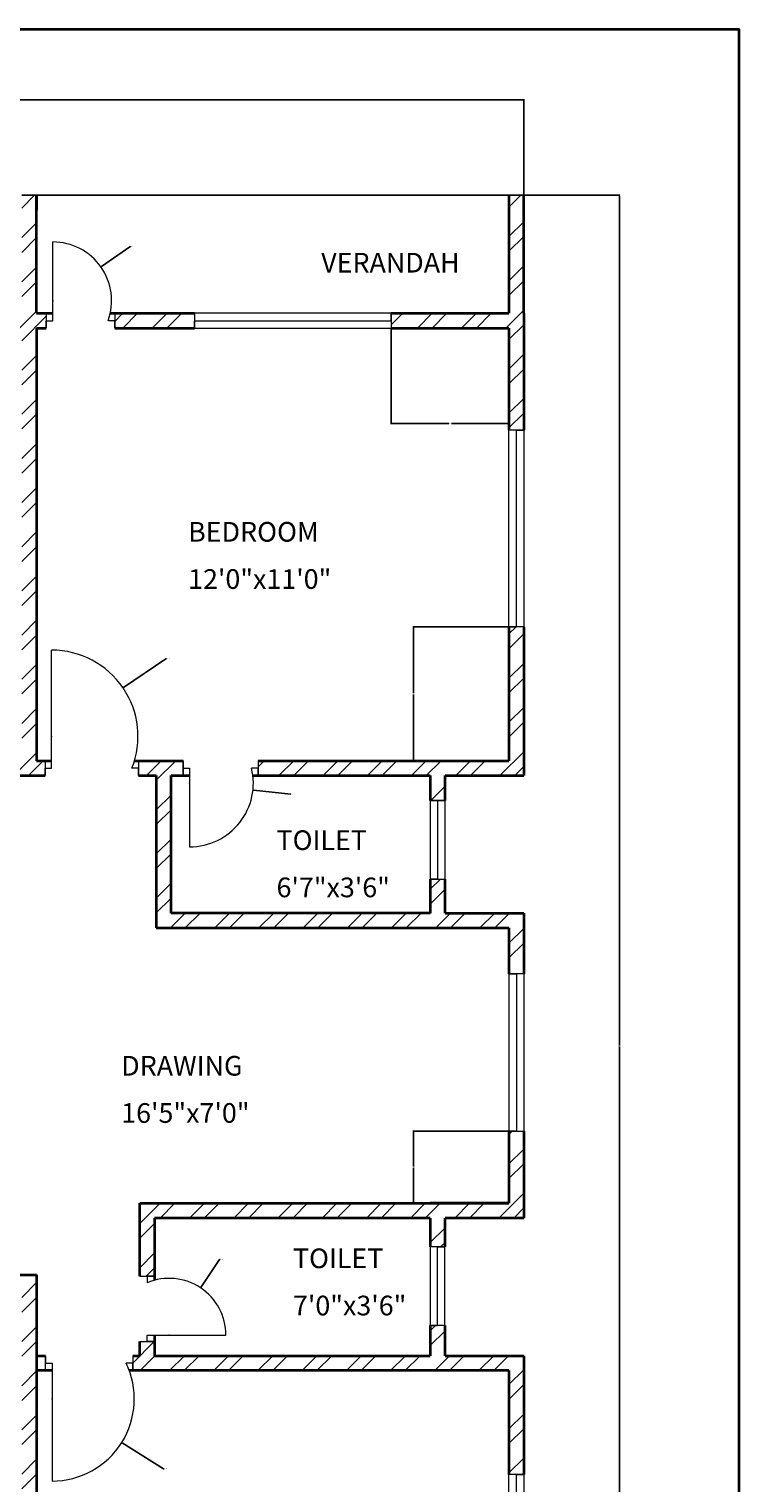
# Model space of a CAD drawing. Units: inches. Extents: x 2271 to 2815, y 1169 to 1838.
# Tile 4 of 4: x 2599 to 2815, y 1395 to 1838. Entities that reach past the tile are written whole.
import ezdxf

# ---------------------------------------------------------------- set-up
doc = ezdxf.new("R2010")
doc.units = ezdxf.units.IN
for name, color, linetype, lineweight in [('A-ANNO-DIMS', 2, 'Continuous', 18), ('A-ANNO-TTLB', 7, 'Continuous', 35), ('A-AREA-IDEN', 7, 'Continuous', 18), ('A-DOOR', 11, 'Continuous', 18), ('A-FLOR-EDGE', 7, 'Continuous', 25), ('A-GLAZ', 181, 'Continuous', 18), ('A-WALL', 7, 'Continuous', 35)]:
    doc.layers.add(name, color=color, linetype=linetype, lineweight=lineweight)
doc.layers.add('A-WALL-PATT', color=9, linetype='Continuous', lineweight=13, true_color=0xafd9aa)
doc.styles.get("Standard").update_dxf_attribs({"font": 'arial.ttf'})
doc.dimstyles.get("Standard").update_dxf_attribs({"dimtxt": 0.18, "dimasz": 0.18, "dimexe": 0.18, "dimexo": 0.0625, "dimgap": 0.09, "dimtad": 0, "dimtih": 1, "dimtoh": 1, "dimdec": 4, "dimzin": 0, "dimdsep": 46, "dimtxsty": 'Standard', "dimcen": 0.09, "dimadec": 0, "dimazin": 0, "dimtfac": 1, "dimtdec": 4, "dimtofl": 0, "dimtmove": 0, "dimatfit": 3, "dimfxl": 1, "dimtolj": 1, "dimtzin": 0, "dimarcsym": 0})

# ---------------------------------------------------------------- blocks, each defined once
blk = doc.blocks.new('WIN-60IN')
for p, q in [((0, 4.5), (0, 0)), ((60, 4.5), (0, 4.5)), ((60, 2.25), (60, 4.5)), ((60, 4.5), (60, 0)), ((0, 0), (0, 2.25)), ((0, 2.25), (60, 2.25)), ((0, 0), (60, 0))]:
    blk.add_line(p, q)
blk = doc.blocks.new('WIN-24IN')
for p, q in [((0, 4.5), (0, 0)), ((0, 4.5), (24, 4.5)), ((24, 2.25), (24, 4.5)), ((24, 4.5), (24, 0)), ((0, 0), (0, 2.25)), ((0, 2.25), (24, 2.25)), ((24, 0), (0, 0))]:
    blk.add_line(p, q)
blk = doc.blocks.new('*D7')
at = {"layer": 'A-ANNO-DIMS', "color": 0, "lineweight": -2, "transparency": 16777216}
for p, q in [((2318.8, 1787.59), (2318.8, 1816.86)), ((2318.98, 1816.68), (2533.65, 1816.68)), ((2749.12, 1816.68), (2534.45, 1816.68)), ((2749.3, 1787.59), (2749.3, 1816.86))]:
    blk.add_line(p, q, dxfattribs=at)
at = {"layer": 'A-ANNO-DIMS', "color": 0, "transparency": 16777216}
for points in [[(2318.98, 1816.71), (2318.98, 1816.65), (2318.8, 1816.68)], [(2749.12, 1816.71), (2749.12, 1816.65), (2749.3, 1816.68)]]:
    blk.add_solid(points, dxfattribs=at)
at = {"layer": 'Defpoints', "color": 0, "transparency": 16777216}
for p in [(2749.3, 1816.68), (2318.8, 1787.53), (2749.3, 1787.53)]:
    blk.add_point(p, dxfattribs=at)
at = {"layer": 'A-ANNO-DIMS', "color": 0, "transparency": 16777216, "insert": (2534.05, 1816.68), "char_height": 0.18, "attachment_point": 5}
blk.add_mtext('\\A1;430.5', dxfattribs=at)
blk = doc.blocks.new('*D8')
at = {"layer": 'A-ANNO-DIMS', "color": 0, "lineweight": -2, "transparency": 16777216}
for p, q in [((2749.36, 1787.53), (2778.63, 1787.53)), ((2778.45, 1787.35), (2778.45, 1528.21)), ((2778.45, 1268.71), (2778.45, 1527.85)), ((2749.36, 1268.53), (2778.63, 1268.53))]:
    blk.add_line(p, q, dxfattribs=at)
at = {"layer": 'A-ANNO-DIMS', "color": 0, "transparency": 16777216}
for points in [[(2778.42, 1787.35), (2778.48, 1787.35), (2778.45, 1787.53)], [(2778.42, 1268.71), (2778.48, 1268.71), (2778.45, 1268.53)]]:
    blk.add_solid(points, dxfattribs=at)
at = {"layer": 'Defpoints', "color": 0, "transparency": 16777216}
for p in [(2749.3, 1787.53), (2778.45, 1787.53), (2749.3, 1268.53)]:
    blk.add_point(p, dxfattribs=at)
at = {"layer": 'A-ANNO-DIMS', "color": 0, "transparency": 16777216, "insert": (2778.45, 1528.03), "char_height": 0.18, "attachment_point": 5}
blk.add_mtext('\\A1;519', dxfattribs=at)
blk = doc.blocks.new('*D29')
at = {"layer": 'A-ANNO-DIMS', "color": 0, "lineweight": -2, "transparency": 16777216}
for p, q in [((2708.93, 1746.97), (2708.93, 1717.7)), ((2744.8, 1746.97), (2744.8, 1717.7)), ((2709.11, 1717.88), (2726.47, 1717.88)), ((2744.62, 1717.88), (2727.26, 1717.88))]:
    blk.add_line(p, q, dxfattribs=at)
at = {"layer": 'A-ANNO-DIMS', "color": 0, "transparency": 16777216}
for points in [[(2709.11, 1717.91), (2709.11, 1717.85), (2708.93, 1717.88)], [(2744.62, 1717.91), (2744.62, 1717.85), (2744.8, 1717.88)]]:
    blk.add_solid(points, dxfattribs=at)
at = {"layer": 'Defpoints', "color": 0, "transparency": 16777216}
for p in [(2708.93, 1747.03), (2744.8, 1747.03), (2708.93, 1717.88)]:
    blk.add_point(p, dxfattribs=at)
at = {"layer": 'A-ANNO-DIMS', "color": 0, "transparency": 16777216, "insert": (2726.87, 1717.88), "char_height": 0.18, "attachment_point": 5}
blk.add_mtext('\\A1;35.87', dxfattribs=at)
blk = doc.blocks.new('*D34')
at = {"layer": 'A-ANNO-DIMS', "color": 0, "lineweight": -2, "transparency": 16777216}
for p, q in [((2744.74, 1655.86), (2715.47, 1655.86)), ((2715.65, 1655.68), (2715.65, 1635.63)), ((2715.65, 1615.21), (2715.65, 1635.26)), ((2744.74, 1615.03), (2715.47, 1615.03))]:
    blk.add_line(p, q, dxfattribs=at)
at = {"layer": 'A-ANNO-DIMS', "color": 0, "transparency": 16777216}
for points in [[(2715.62, 1655.68), (2715.68, 1655.68), (2715.65, 1655.86)], [(2715.62, 1615.21), (2715.68, 1615.21), (2715.65, 1615.03)]]:
    blk.add_solid(points, dxfattribs=at)
at = {"layer": 'Defpoints', "color": 0, "transparency": 16777216}
for p in [(2715.65, 1655.86), (2744.8, 1655.86), (2744.8, 1615.03)]:
    blk.add_point(p, dxfattribs=at)
at = {"layer": 'A-ANNO-DIMS', "color": 0, "transparency": 16777216, "insert": (2715.65, 1635.44), "char_height": 0.18, "attachment_point": 5}
blk.add_mtext('\\A1;40.826', dxfattribs=at)
blk = doc.blocks.new('*D35')
at = {"layer": 'A-ANNO-DIMS', "color": 0, "lineweight": -2, "transparency": 16777216}
for p, q in [((2744.74, 1502.04), (2715.47, 1502.04)), ((2715.65, 1501.86), (2715.65, 1491.22)), ((2715.65, 1480.21), (2715.65, 1490.85)), ((2744.74, 1480.03), (2715.47, 1480.03))]:
    blk.add_line(p, q, dxfattribs=at)
at = {"layer": 'A-ANNO-DIMS', "color": 0, "transparency": 16777216}
for points in [[(2715.62, 1501.86), (2715.68, 1501.86), (2715.65, 1502.04)], [(2715.62, 1480.21), (2715.68, 1480.21), (2715.65, 1480.03)]]:
    blk.add_solid(points, dxfattribs=at)
at = {"layer": 'Defpoints', "color": 0, "transparency": 16777216}
for p in [(2715.65, 1502.04), (2744.8, 1502.04), (2744.8, 1480.03)]:
    blk.add_point(p, dxfattribs=at)
at = {"layer": 'A-ANNO-DIMS', "color": 0, "transparency": 16777216, "insert": (2715.65, 1491.04), "char_height": 0.18, "attachment_point": 5}
blk.add_mtext('\\A1;22.01', dxfattribs=at)
blk = doc.blocks.new('*D40')
at = {"layer": 'A-ANNO-DIMS', "color": 0, "lineweight": -2, "transparency": 16777216}
for p, q in [((2640.24, 1646.14), (2627.33, 1637.36)), ((2640.42, 1646.14), (2640.24, 1646.14)), ((2605.33, 1622.46), (2605.51, 1622.46)), ((2605.42, 1622.37), (2605.42, 1622.55))]:
    blk.add_line(p, q, dxfattribs=at)
at = {"layer": 'A-ANNO-DIMS', "color": 0, "transparency": 16777216}
blk.add_solid([(2627.31, 1637.39), (2627.35, 1637.34), (2627.18, 1637.26)], dxfattribs=at)
at = {"layer": 'Defpoints', "color": 0, "transparency": 16777216}
for p in [(2627.18, 1637.26), (2605.42, 1622.46)]:
    blk.add_point(p, dxfattribs=at)
at = {"layer": 'A-ANNO-DIMS', "color": 0, "transparency": 16777216, "insert": (2640.9, 1646.14), "char_height": 0.18, "attachment_point": 5}
blk.add_mtext('\\A1;R26.32', dxfattribs=at)
blk = doc.blocks.new('*D42')
at = {"layer": 'A-ANNO-DIMS', "color": 0, "lineweight": -2, "transparency": 16777216}
for p, q in [((2605.45, 1420.36), (2605.63, 1420.36)), ((2605.54, 1420.27), (2605.54, 1420.45)), ((2639.53, 1399.04), (2626.94, 1406.94)), ((2639.71, 1399.04), (2639.53, 1399.04))]:
    blk.add_line(p, q, dxfattribs=at)
at = {"layer": 'A-ANNO-DIMS', "color": 0, "transparency": 16777216}
blk.add_solid([(2626.95, 1406.97), (2626.92, 1406.92), (2626.78, 1407.04)], dxfattribs=at)
at = {"layer": 'Defpoints', "color": 0, "transparency": 16777216}
for p in [(2605.54, 1420.36), (2626.78, 1407.04)]:
    blk.add_point(p, dxfattribs=at)
at = {"layer": 'A-ANNO-DIMS', "color": 0, "transparency": 16777216, "insert": (2640.19, 1399.04), "char_height": 0.18, "attachment_point": 5}
blk.add_mtext('\\A1;R25.08', dxfattribs=at)
blk = doc.blocks.new('*D44')
at = {"layer": 'A-ANNO-DIMS', "color": 0, "lineweight": -2, "transparency": 16777216}
for p, q in [((2647.39, 1608.19), (2647.57, 1608.19)), ((2647.48, 1608.1), (2647.48, 1608.28)), ((2678.36, 1604.85), (2666.96, 1606.08))]:
    blk.add_line(p, q, dxfattribs=at)
at = {"layer": 'A-ANNO-DIMS', "color": 0, "transparency": 16777216}
blk.add_solid([(2666.96, 1606.11), (2666.96, 1606.05), (2666.78, 1606.1)], dxfattribs=at)
at = {"layer": 'Defpoints', "color": 0, "transparency": 16777216}
for p in [(2647.48, 1608.19), (2666.78, 1606.1)]:
    blk.add_point(p, dxfattribs=at)
at = {"layer": 'A-ANNO-DIMS', "color": 0, "transparency": 16777216, "insert": (2678.91, 1604.85), "char_height": 0.18, "attachment_point": 5}
blk.add_mtext('\\A1;R19.413', dxfattribs=at)
blk = doc.blocks.new('*D48')
at = {"layer": 'A-ANNO-DIMS', "color": 0, "lineweight": -2, "transparency": 16777216}
for p, q in [((2629.25, 1771.84), (2620.6, 1765.76)), ((2629.43, 1771.84), (2629.25, 1771.84)), ((2605.7, 1755.37), (2605.88, 1755.37)), ((2605.79, 1755.28), (2605.79, 1755.46))]:
    blk.add_line(p, q, dxfattribs=at)
at = {"layer": 'A-ANNO-DIMS', "color": 0, "transparency": 16777216}
blk.add_solid([(2620.58, 1765.79), (2620.62, 1765.74), (2620.45, 1765.66)], dxfattribs=at)
at = {"layer": 'Defpoints', "color": 0, "transparency": 16777216}
for p in [(2620.45, 1765.66), (2605.79, 1755.37)]:
    blk.add_point(p, dxfattribs=at)
at = {"layer": 'A-ANNO-DIMS', "color": 0, "transparency": 16777216, "insert": (2629.98, 1771.84), "char_height": 0.18, "attachment_point": 5}
blk.add_mtext('\\A1;R17.915', dxfattribs=at)
blk = doc.blocks.new('*D50')
at = {"layer": 'A-ANNO-DIMS', "color": 0, "lineweight": -2, "transparency": 16777216}
for p, q in [((2656.58, 1462.88), (2650.93, 1454.39)), ((2656.76, 1462.88), (2656.58, 1462.88)), ((2641.16, 1439.83), (2641.34, 1439.83)), ((2641.25, 1439.74), (2641.25, 1439.92))]:
    blk.add_line(p, q, dxfattribs=at)
at = {"layer": 'A-ANNO-DIMS', "color": 0, "transparency": 16777216}
blk.add_solid([(2650.9, 1454.41), (2650.95, 1454.37), (2650.83, 1454.24)], dxfattribs=at)
at = {"layer": 'Defpoints', "color": 0, "transparency": 16777216}
for p in [(2650.83, 1454.24), (2641.25, 1439.83)]:
    blk.add_point(p, dxfattribs=at)
at = {"layer": 'A-ANNO-DIMS', "color": 0, "transparency": 16777216, "insert": (2657.3, 1462.88), "char_height": 0.18, "attachment_point": 5}
blk.add_mtext('\\A1;R17.304', dxfattribs=at)

msp = doc.modelspace()

# ---------------------------------------------------------------- hatches: boundary and pattern name
at = {"layer": 'A-WALL-PATT'}
h = msp.add_hatch(dxfattribs=at)
h.set_pattern_fill('ANSI32', color=256)
h.paths.add_polyline_path([(2441.4917, 1751.5314), (2397.0578, 1751.5314), (2397.0578, 1747.0314), (2441.4917, 1747.0314), (2441.4917, 1749.2814)])
h.paths.add_polyline_path([(2471.8006, 1787.5314), (2467.3006, 1787.5314), (2467.3006, 1783.0314), (2467.3006, 1751.5314), (2463.4131, 1751.5314), (2463.4131, 1747.0314), (2467.3006, 1747.0314), (2467.3006, 1615.0314), (2465.0606, 1615.0314), (2465.0606, 1610.5314), (2474.7192, 1610.5314), (2474.7192, 1612.7814), (2474.7192, 1615.0314), (2471.8006, 1615.0314), (2471.8006, 1747.0314), (2482.8275, 1747.0314), (2482.8275, 1749.2814), (2482.8275, 1751.5314), (2471.8006, 1751.5314)])
h.paths.add_polyline_path([(2549.5185, 1751.5314), (2506.8275, 1751.5314), (2506.8275, 1747.0314), (2531.8006, 1747.0314), (2531.8006, 1615.0314), (2496.0724, 1615.0314), (2496.0724, 1610.5314), (2531.8006, 1610.5314), (2531.8006, 1458.2548), (2528.7405, 1458.2548), (2528.7405, 1453.7548), (2539.7806, 1453.7548), (2539.7806, 1456.0048), (2539.7806, 1458.2548), (2536.3006, 1458.2548), (2536.3006, 1610.5314), (2573.267, 1610.5314), (2573.267, 1612.5736), (2573.267, 1612.7912), (2573.267, 1615.0314), (2536.3006, 1615.0314), (2536.3006, 1747.0314), (2549.5185, 1747.0314)])
h.paths.add_polyline_path([(2600.8006, 1787.5314), (2596.3006, 1787.5314), (2596.3006, 1747.0314), (2596.3006, 1615.0314), (2593.1473, 1615.0314), (2593.1473, 1610.5314), (2603.416, 1610.5314), (2603.416, 1612.7814), (2603.416, 1615.0314), (2600.8006, 1615.0314), (2600.8006, 1747.0314), (2603.7892, 1747.0314), (2603.7892, 1749.2814), (2603.7892, 1751.5314), (2600.8006, 1751.5314)])
h.paths.add_polyline_path([(2596.3006, 1751.5314), (2573.5185, 1751.5314), (2573.5185, 1747.0314), (2596.3006, 1747.0314)])
h.paths.add_polyline_path([(2648.9302, 1749.2814), (2648.9302, 1751.5314), (2624.6394, 1751.5314), (2624.6394, 1747.0314), (2648.9302, 1747.0314)])
h.paths.add_polyline_path([(2749.3006, 1751.5314), (2749.3006, 1787.5314), (2744.8006, 1787.5314), (2744.8006, 1751.5314), (2708.9302, 1751.5314), (2708.9302, 1747.0314), (2744.8006, 1747.0314), (2744.8006, 1715.8571), (2749.3006, 1715.8571)])
h.paths.add_polyline_path([(2337.0578, 1749.2814), (2337.0578, 1751.5314), (2323.3006, 1751.5314), (2323.3006, 1787.5314), (2318.8006, 1787.5314), (2318.8006, 1751.5314), (2318.8006, 1712.2179), (2323.3006, 1712.2179), (2323.3006, 1747.0314), (2337.0578, 1747.0314)])
h.paths.add_polyline_path([(2402.757, 1615.0314), (2323.3006, 1615.0314), (2323.3006, 1652.2179), (2318.8006, 1652.2179), (2318.8006, 1610.5314), (2323.3006, 1610.5314), (2342.8006, 1610.5314), (2342.8006, 1602.42), (2347.3006, 1602.42), (2347.3006, 1610.5314), (2402.757, 1610.5314)])
h.paths.add_polyline_path([(2430.8006, 1568.5314), (2430.8006, 1610.5314), (2434.8435, 1610.5314), (2434.8435, 1612.7814), (2434.8435, 1615.0314), (2422.3947, 1615.0314), (2422.3947, 1612.7814), (2422.3947, 1610.5314), (2426.3006, 1610.5314), (2426.3006, 1568.5314), (2347.3006, 1568.5314), (2347.3006, 1578.42), (2342.8006, 1578.42), (2342.8006, 1568.5314), (2318.8006, 1568.5314), (2318.8006, 1546.0693), (2322.7121, 1546.0693), (2323.3006, 1546.0693), (2323.3006, 1564.0314), (2342.8006, 1564.0314), (2347.3006, 1564.0314), (2430.8006, 1564.0314)])
h.paths.add_polyline_path([(2430.8006, 1480.0314), (2323.3006, 1480.0314), (2323.3006, 1498.0693), (2321.0506, 1498.0693), (2318.8006, 1498.0693), (2318.8006, 1475.5314), (2342.8006, 1475.5314), (2342.8006, 1466.8218), (2347.3006, 1466.8218), (2347.3006, 1475.5314), (2426.3006, 1475.5314), (2426.3006, 1458.0149), (2430.8006, 1458.0149), (2430.8006, 1475.5314)])
h.paths.add_polyline_path([(2435.9471, 1433.5314), (2430.8006, 1433.5314), (2430.8006, 1437.7896), (2426.3006, 1437.7896), (2426.3006, 1433.5314), (2347.3006, 1433.5314), (2347.3006, 1442.8218), (2342.8006, 1442.8218), (2342.8006, 1433.5314), (2318.8006, 1433.5314), (2318.8006, 1402.3145), (2323.3006, 1402.3145), (2323.3006, 1429.0314), (2342.8006, 1429.0314), (2347.3006, 1429.0314), (2435.9471, 1429.0314)])
h.paths.add_polyline_path([(2323.3006, 1342.3145), (2321.0506, 1342.3145), (2318.8006, 1342.3145), (2318.8006, 1304.5314), (2318.8006, 1268.5314), (2323.3006, 1268.5314), (2323.3006, 1304.5314), (2333.4662, 1304.5314), (2333.4662, 1306.7814), (2333.4662, 1309.0314), (2323.3006, 1309.0314)])
h.paths.add_polyline_path([(2437.8933, 1306.7814), (2437.8933, 1309.0314), (2393.4662, 1309.0314), (2393.4662, 1304.5314), (2437.8933, 1304.5314)])
h.paths.add_polyline_path([(2471.8006, 1453.7548), (2493.7895, 1453.7548), (2493.7895, 1456.0048), (2493.7895, 1458.2548), (2467.3006, 1458.2548), (2467.3006, 1433.5314), (2463.7134, 1433.5314), (2463.7134, 1431.2814), (2463.7134, 1429.0314), (2467.3006, 1429.0314), (2467.3006, 1309.0314), (2462.3197, 1309.0314), (2462.3197, 1304.5314), (2467.3006, 1304.5314), (2467.3006, 1268.5314), (2471.8006, 1268.5314), (2495.9201, 1268.5314), (2495.9201, 1270.7814), (2495.9201, 1273.0314), (2471.8006, 1273.0314), (2471.8006, 1309.0314)])
h.paths.add_polyline_path([(2600.8006, 1458.2548), (2570.4818, 1458.2548), (2570.4818, 1453.7548), (2596.3006, 1453.7548), (2596.3006, 1429.0314), (2596.3006, 1273.0314), (2555.9201, 1273.0314), (2555.9201, 1268.5314), (2596.3006, 1268.5314), (2600.8006, 1268.5314), (2600.8006, 1304.5314), (2604.5593, 1304.5314), (2604.5593, 1306.7814), (2604.5593, 1309.0314), (2600.8006, 1309.0314), (2600.8006, 1429.0314)])
h.paths.add_polyline_path([(2667.0861, 1309.0314), (2627.2, 1309.0314), (2627.2, 1304.5314), (2667.0861, 1304.5314)])
h.paths.add_polyline_path([(2749.3006, 1309.0314), (2749.3006, 1337.3095), (2744.8006, 1337.3095), (2744.8006, 1309.0314), (2727.0861, 1309.0314), (2727.0861, 1306.7814), (2727.0861, 1304.5314), (2744.8006, 1304.5314), (2744.8006, 1268.5314), (2749.3006, 1268.5314), (2749.3006, 1304.5314)])
h.paths.add_polyline_path([(2749.3006, 1433.5314), (2725.3006, 1433.5314), (2725.3006, 1442.7202), (2720.8006, 1442.7202), (2720.8006, 1433.5314), (2636.8006, 1433.5314), (2636.8006, 1437.8287), (2634.5506, 1437.8287), (2632.3006, 1437.8287), (2632.3006, 1433.5314), (2630.1129, 1433.5314), (2630.1129, 1429.0314), (2744.8006, 1429.0314), (2744.8006, 1397.3095), (2749.3006, 1397.3095)])
h.paths.add_polyline_path([(2749.3006, 1480.0314), (2749.3006, 1502.0415), (2744.8006, 1502.0415), (2744.8006, 1480.0314), (2720.8006, 1480.0314), (2632.3006, 1480.0314), (2632.3006, 1457.7851), (2636.8006, 1457.7851), (2636.8006, 1475.5314), (2720.8006, 1475.5314), (2720.8006, 1466.7202), (2725.3006, 1466.7202), (2725.3006, 1475.5314), (2749.3006, 1475.5314)])
h.paths.add_polyline_path([(2749.3006, 1568.5314), (2725.3006, 1568.5314), (2725.3006, 1578.9125), (2720.8006, 1578.9125), (2720.8006, 1568.5314), (2641.8006, 1568.5314), (2641.8006, 1610.5314), (2645.4823, 1610.5314), (2645.4823, 1612.7814), (2645.4823, 1615.0314), (2631.895, 1615.0314), (2631.895, 1610.5314), (2637.3006, 1610.5314), (2637.3006, 1568.5314), (2637.3006, 1564.0314), (2720.8006, 1564.0314), (2725.3006, 1564.0314), (2744.8006, 1564.0314), (2744.8006, 1550.0415), (2747.0506, 1550.0415), (2749.3006, 1550.0415)])
h.paths.add_polyline_path([(2749.3006, 1655.8571), (2744.8006, 1655.8571), (2744.8006, 1615.0314), (2668.3453, 1615.0314), (2668.3453, 1610.5314), (2720.8006, 1610.5314), (2720.8006, 1602.9125), (2725.3006, 1602.9125), (2725.3006, 1610.5314), (2749.3006, 1610.5314)])
h.paths.add_polyline_path([(2512.9815, 1676.2212), (2512.9815, 1716.3099), (2486.1477, 1716.3099), (2486.1477, 1676.2212)], flags=9)

# ---------------------------------------------------------------- linework, layer by layer
at = {"layer": 'A-ANNO-TTLB'}
msp.add_lwpolyline([(2270.5512, 1838.2339), (2814.8691, 1838.2339), (2814.8691, 1168.8883), (2270.5512, 1168.8883)], close=True, dxfattribs=at)
at = {"layer": 'A-DOOR'}
for p, q in [((2605.7892, 1749.2814), (2605.7892, 1773.2814)), ((2603.7892, 1751.5314), (2603.7892, 1747.0314)), ((2603.7892, 1747.0314), (2603.7892, 1749.2814)), ((2603.7892, 1749.2814), (2605.7892, 1749.2814)), ((2624.6394, 1749.2814), (2622.6394, 1749.2814)), ((2624.6394, 1751.5314), (2624.6394, 1747.0314)), ((2624.6394, 1747.0314), (2624.6394, 1749.2814)), ((2605.416, 1612.7814), (2605.416, 1648.7814)), ((2603.416, 1615.0314), (2603.416, 1610.5314)), ((2631.895, 1615.0314), (2631.895, 1610.5314)), ((2645.4823, 1610.5314), (2645.4823, 1615.0314)), ((2645.4823, 1615.0314), (2645.4823, 1610.5314)), ((2668.3453, 1615.0314), (2668.3453, 1610.5314)), ((2603.416, 1610.5314), (2603.416, 1612.7814)), ((2603.416, 1612.7814), (2605.416, 1612.7814)), ((2631.895, 1612.7814), (2629.895, 1612.7814)), ((2631.895, 1610.5314), (2631.895, 1612.7814)), ((2645.4823, 1610.5314), (2645.4823, 1612.7814)), ((2645.4823, 1612.7814), (2647.4823, 1612.7814)), ((2647.4823, 1612.7814), (2647.4823, 1588.7814)), ((2668.3453, 1612.7814), (2666.3453, 1612.7814)), ((2668.3453, 1610.5314), (2668.3453, 1612.7814)), ((2632.3006, 1457.7851), (2636.8006, 1457.7851)), ((2636.8006, 1457.7851), (2634.5506, 1457.7851)), ((2634.5506, 1457.7851), (2634.5506, 1455.7851)), ((2632.3006, 1437.8287), (2636.8006, 1437.8287)), ((2634.5506, 1437.8287), (2634.5506, 1439.8287)), ((2634.5506, 1439.8287), (2658.5506, 1439.8287)), ((2636.8006, 1437.8287), (2634.5506, 1437.8287)), ((2603.5387, 1429.0314), (2603.5387, 1433.5314)), ((2603.5387, 1433.5314), (2603.5387, 1431.2814)), ((2630.1129, 1433.5314), (2630.1129, 1429.0314)), ((2603.5387, 1431.2814), (2605.5387, 1431.2814)), ((2605.5387, 1431.2814), (2605.5387, 1395.2814)), ((2630.1129, 1431.2814), (2628.1129, 1431.2814)), ((2630.1129, 1429.0314), (2630.1129, 1431.2814))]:
    msp.add_line(p, q, dxfattribs=at)
for centre, radius, start, end in [((2605.7892, 1755.3662), 17.9152, 340.144636, 90), ((2605.416, 1622.4589), 26.3225, 338.429293, 90), ((2647.4823, 1608.1941), 19.4127, 270, 13.668434), ((2641.2463, 1439.8287), 17.3043, 0, 112.764112), ((2605.5387, 1420.3591), 25.0777, 270, 25.819443)]:
    msp.add_arc(centre, radius, start, end, dxfattribs=at)
at = {"layer": 'A-FLOR-EDGE'}
msp.add_line((2749.3006, 1787.5314), (2596.3006, 1787.5314), dxfattribs=at)
at = {"layer": 'A-GLAZ'}
for p, q in [((2725.3006, 1602.9125), (2720.8006, 1602.9125)), ((2720.8006, 1602.9125), (2725.3006, 1602.9125)), ((2720.8006, 1602.9125), (2720.8006, 1578.9125)), ((2725.3006, 1602.9125), (2723.0506, 1602.9125)), ((2723.0506, 1602.9125), (2723.0506, 1578.9125)), ((2725.3006, 1578.9125), (2725.3006, 1602.9125)), ((2723.0506, 1578.9125), (2720.8006, 1578.9125)), ((2720.8006, 1578.9125), (2725.3006, 1578.9125)), ((2749.3006, 1550.0415), (2744.8006, 1550.0415)), ((2744.8006, 1550.0415), (2747.0506, 1550.0415)), ((2744.8006, 1550.0415), (2744.8006, 1502.0415)), ((2747.0506, 1550.0415), (2747.0506, 1502.0415)), ((2749.3006, 1550.0415), (2749.3006, 1502.0415)), ((2747.0506, 1502.0415), (2744.8006, 1502.0415)), ((2744.8006, 1502.0415), (2749.3006, 1502.0415))]:
    msp.add_line(p, q, dxfattribs=at)
at = {"layer": 'A-WALL'}
for p, q in [((2600.8006, 1751.5314), (2600.8006, 1787.5314)), ((2600.8006, 1787.5314), (2600.8006, 1783.0314)), ((2744.8006, 1787.5314), (2744.8006, 1751.5314)), ((2749.3006, 1751.5314), (2749.3006, 1787.5314)), ((2600.8006, 1751.5314), (2605.7892, 1751.5314)), ((2623.2892, 1751.5314), (2648.9302, 1751.5314)), ((2708.9302, 1751.5314), (2744.8006, 1751.5314)), ((2749.3006, 1751.5314), (2749.3006, 1715.8571)), ((2600.8006, 1747.0314), (2600.8006, 1615.0314)), ((2600.8006, 1747.0314), (2603.7892, 1747.0314)), ((2624.6394, 1747.0314), (2648.9302, 1747.0314)), ((2708.9302, 1747.0314), (2744.8006, 1747.0314)), ((2744.8006, 1747.0314), (2744.8006, 1715.8571)), ((2744.8006, 1655.8571), (2744.8006, 1615.0314)), ((2749.3006, 1655.8571), (2749.3006, 1610.5314)), ((2600.8006, 1615.0314), (2605.416, 1615.0314)), ((2630.6689, 1615.0314), (2645.4823, 1615.0314)), ((2668.3453, 1615.0314), (2744.8006, 1615.0314)), ((2593.1473, 1610.5314), (2603.416, 1610.5314)), ((2631.895, 1610.5314), (2637.3006, 1610.5314)), ((2637.3006, 1610.5314), (2637.3006, 1568.5314)), ((2641.8006, 1568.5314), (2641.8006, 1610.5314)), ((2641.8006, 1610.5314), (2647.4823, 1610.5314)), ((2666.7538, 1610.5314), (2720.8006, 1610.5314)), ((2720.8006, 1610.5314), (2720.8006, 1602.9125)), ((2720.8006, 1610.5314), (2720.8006, 1602.9125)), ((2725.3006, 1610.5314), (2749.3006, 1610.5314)), ((2725.3006, 1602.9125), (2725.3006, 1610.5314)), ((2720.8006, 1578.9125), (2720.8006, 1568.5314)), ((2720.8006, 1578.9125), (2720.8006, 1568.5314)), ((2725.3006, 1568.5314), (2725.3006, 1578.9125)), ((2637.3006, 1568.5314), (2637.3006, 1564.0314)), ((2720.8006, 1568.5314), (2641.8006, 1568.5314)), ((2725.3006, 1568.5314), (2749.3006, 1568.5314)), ((2749.3006, 1568.5314), (2749.3006, 1550.0415)), ((2637.3006, 1564.0314), (2720.8006, 1564.0314)), ((2720.8006, 1564.0314), (2720.8006, 1564.0314)), ((2720.8006, 1564.0314), (2725.3006, 1564.0314)), ((2725.3006, 1564.0314), (2744.8006, 1564.0314)), ((2744.8006, 1564.0314), (2744.8006, 1550.0415)), ((2744.8006, 1502.0415), (2744.8006, 1480.0314)), ((2749.3006, 1502.0415), (2749.3006, 1475.5314)), ((2632.3006, 1480.0314), (2744.8006, 1480.0314)), ((2632.3006, 1457.7851), (2632.3006, 1480.0314)), ((2744.8006, 1480.0314), (2720.8006, 1480.0314)), ((2749.3006, 1480.0314), (2749.3006, 1475.5314)), ((2720.8006, 1475.5314), (2636.8006, 1475.5314)), ((2636.8006, 1475.5314), (2636.8006, 1456.5521)), ((2720.8006, 1475.5314), (2720.8006, 1466.7202)), ((2749.3006, 1475.5314), (2725.3006, 1475.5314)), ((2725.3006, 1466.7202), (2725.3006, 1475.5314)), ((2569.063, 1458.2548), (2600.8006, 1458.2548)), ((2600.8006, 1458.2548), (2600.8006, 1429.0314)), ((2720.8006, 1442.7202), (2720.8006, 1433.5314)), ((2725.3006, 1433.5314), (2725.3006, 1442.7202)), ((2632.3006, 1433.5314), (2632.3006, 1437.8287)), ((2636.8006, 1439.8287), (2636.8006, 1433.5314)), ((2600.8006, 1433.5314), (2603.5387, 1433.5314)), ((2630.1129, 1433.5314), (2632.3006, 1433.5314)), ((2636.8006, 1433.5314), (2720.8006, 1433.5314)), ((2725.3006, 1433.5314), (2749.3006, 1433.5314)), ((2749.3006, 1433.5314), (2749.3006, 1397.3095)), ((2600.8006, 1429.0314), (2600.8006, 1309.0314)), ((2605.5387, 1429.0314), (2600.8006, 1429.0314)), ((2744.8006, 1429.0314), (2629.0692, 1429.0314)), ((2744.8006, 1429.0314), (2744.8006, 1397.3095))]:
    msp.add_line(p, q, dxfattribs=at)

# ---------------------------------------------------------------- block references
at = {"layer": 'A-GLAZ'}
msp.add_blockref('WIN-60IN', (2648.9304, 1747.031), dxfattribs=at)
at = {"layer": 'A-GLAZ', "extrusion": (0, 0, -1), "zscale": -1, "rotation": 90}
for name, p in [('WIN-60IN', (-2744.8001, 1655.8574)), ('WIN-24IN', (-2720.8001, 1442.7197)), ('WIN-60IN', (-2744.8001, 1337.3097))]:
    msp.add_blockref(name, p, dxfattribs=at)

# ---------------------------------------------------------------- texts
at = {"layer": 'A-AREA-IDEN', "char_height": 6, "attachment_point": 1, "line_spacing_factor": 1.44}
for s, width, insert in [('VERANDAH', 202.405664, (2687.575, 1769.9702)), ('BEDROOM\\P12\'0"x11\'0"', 179.913428, (2647.0138, 1687.8673)), ('TOILET\\P6\'7"x3\'6"', 107.029993, (2673.9563, 1593.799)), ('DRAWING\\P16\'5"x7\'0"', 153.715954, (2626.6242, 1524.9791)), ('TOILET\\P7\'0"x3\'6"', 88.023145, (2678.9695, 1466.2427))]:
    msp.add_mtext_dynamic_manual_height_columns(s, width=width, gutter_width=12.5, heights=[0], dxfattribs=dict(at, insert=insert))

# ---------------------------------------------------------------- dimensions: what is measured, and where the dimension line sits
at = {"layer": 'A-ANNO-DIMS'}
dim = msp.add_linear_dim(base=(2749.3006, 1816.6814), p1=(2318.8006, 1787.5314), p2=(2749.3006, 1787.5314), dimstyle='Standard', override={"dimdec": 1, "dimlfac": 1, "dimrnd": 0, "dimzin": 0, "dimdsep": 46, "dimlunit": 2}, dxfattribs=at)
dim.commit()
dim.dimension.update_dxf_attribs({"geometry": '*D7', "text_midpoint": (2534.0506, 1816.6814)})
for base, p1, p2, angle, override, picture, middle in [((2778.4506, 1787.5314), (2749.3006, 1268.5314), (2749.3006, 1787.5314), 90, {"dimdec": 0, "dimlfac": 1, "dimrnd": 0, "dimzin": 0, "dimdsep": 46, "dimlunit": 2}, '*D8', (2778.4506, 1528.0314)), ((2708.9302, 1717.8814), (2744.8006, 1747.0314), (2708.9302, 1747.0314), 180, {"dimdec": 2, "dimlfac": 1, "dimrnd": 0, "dimzin": 0, "dimdsep": 46, "dimlunit": 2}, '*D29', (2726.8654, 1717.8814)), ((2715.6506, 1655.8571), (2744.8006, 1615.0314), (2744.8006, 1655.8571), 90, {"dimdec": 3, "dimlfac": 1, "dimrnd": 0, "dimzin": 0, "dimdsep": 46, "dimlunit": 2}, '*D34', (2715.6506, 1635.4443)), ((2715.6506, 1502.0415), (2744.8006, 1480.0314), (2744.8006, 1502.0415), 90, {"dimdec": 2, "dimlfac": 1, "dimrnd": 0, "dimzin": 0, "dimdsep": 46, "dimlunit": 2}, '*D35', (2715.6506, 1491.0364))]:
    dim = msp.add_linear_dim(base=base, p1=p1, p2=p2, angle=angle, dimstyle='Standard', override=override, dxfattribs=at)
    dim.commit()
    dim.dimension.update_dxf_attribs({"geometry": picture, "text_midpoint": middle})
for center, mpoint, override, picture, middle in [((2605.7892, 1755.3662), (2620.4516, 1765.6604), {"dimdec": 3, "dimlfac": 1, "dimrnd": 0, "dimzin": 0, "dimdsep": 46, "dimlunit": 2}, '*D48', (2629.9794, 1771.8369)), ((2605.416, 1622.4589), (2627.183, 1637.26), {"dimdec": 2, "dimlfac": 1, "dimrnd": 0, "dimzin": 0, "dimdsep": 46, "dimlunit": 2}, '*D40', (2640.9021, 1646.1407)), ((2647.4823, 1608.1941), (2666.782, 1606.102), {"dimdec": 3, "dimlfac": 1, "dimrnd": 0, "dimzin": 0, "dimdsep": 46, "dimlunit": 2}, '*D44', (2678.3618, 1604.8466)), ((2641.2463, 1439.8287), (2650.8268, 1454.2388), {"dimdec": 3, "dimlfac": 1, "dimrnd": 0, "dimzin": 0, "dimdsep": 46, "dimlunit": 2}, '*D50', (2657.3046, 1462.8848)), ((2605.5387, 1420.3591), (2626.7847, 1407.0362), {"dimdec": 2, "dimlfac": 1, "dimrnd": 0, "dimzin": 0, "dimdsep": 46, "dimlunit": 2}, '*D42', (2640.1923, 1399.0424))]:
    dim = msp.add_radius_dim(center=center, mpoint=mpoint, dimstyle='Standard', override=override, dxfattribs=at)
    dim.commit()
    dim.dimension.update_dxf_attribs({"geometry": picture, "text_midpoint": middle, "dimtype": 164})

doc.saveas('drawing.dxf')
